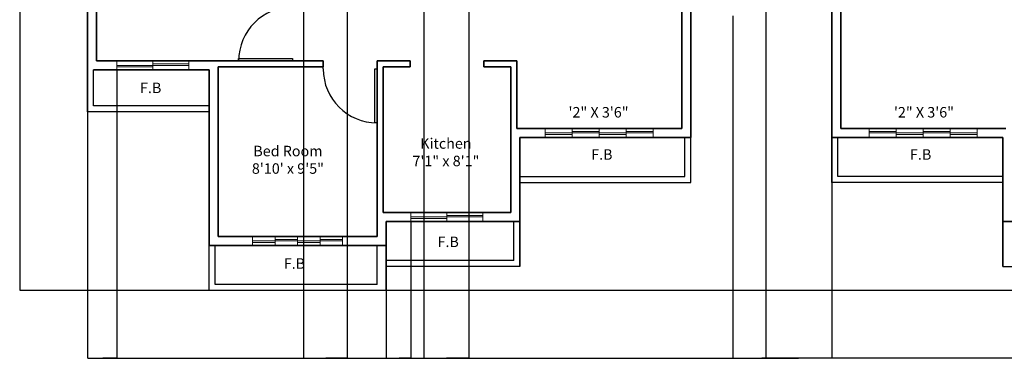
# Model space of a CAD drawing. Units: feet. Extents: x 105 to 1094, y -88 to 588.
# Tile 1 of 59: x 105 to 762, y -88 to 138. Entities that reach past the tile are written whole.
import ezdxf

# ---------------------------------------------------------------- set-up
doc = ezdxf.new("R2010")
doc.units = ezdxf.units.FT
doc.header["$MEASUREMENT"] = 0
for name, color, linetype, lineweight in [('A-ANNO-DIMS', 2, 'Continuous', 18), ('A-ANNO-TEXT', 7, 'Continuous', 18), ('A-AREA-IDEN', 7, 'Continuous', 18), ('A-DOOR', 3, 'Continuous', 25), ('A-FLOR-PROJ', 8, 'Continuous', 25), ('A-GLAZ', 4, 'Continuous', 18), ('A-WALL', 7, 'Continuous', 35)]:
    doc.layers.add(name, color=color, linetype=linetype, lineweight=lineweight)
doc.styles.get("Standard").update_dxf_attribs({"font": 'arial.ttf'})
doc.dimstyles.get("Standard").update_dxf_attribs({"dimtxt": 0.18, "dimasz": 0.18, "dimexe": 0.18, "dimexo": 0.0625, "dimgap": 0.09, "dimtad": 0, "dimtih": 1, "dimtoh": 1, "dimdec": 4, "dimzin": 0, "dimdsep": 46, "dimtxsty": 'Standard', "dimcen": 0.09, "dimadec": 0, "dimazin": 0, "dimtfac": 1, "dimtdec": 4, "dimtofl": 0, "dimtmove": 0, "dimatfit": 3, "dimfxl": 1, "dimtolj": 1, "dimtzin": 0, "dimarcsym": 0})

# ---------------------------------------------------------------- blocks, each defined once
blk = doc.blocks.new('*U2')
for p, q in [((0, 0), (0, -6)), ((40, 0), (40, -6))]:
    blk.add_line(p, q)
blk.add_lwpolyline([(0, 0), (0, 40), (1.75, 40), (1.75, 0)], close=True)
blk.add_arc((0, 0), 40, 0, 90)
blk = doc.blocks.new('WIN-FOUR-LIGHT-WIDE')
for p, q in [((0, 0), (0, 6)), ((0, 3), (72, 3)), ((0, 2), (18, 2)), ((18, 0), (18, 6)), ((18, 4), (36, 4)), ((36, 0), (36, 6)), ((36, 2), (54, 2)), ((54, 0), (54, 6)), ((54, 4), (72, 4)), ((72, 0), (72, 6))]:
    blk.add_line(p, q)
blk = doc.blocks.new('WIN-TWO-LIGHT')
for p, q in [((0, 0), (0, 6)), ((0, 3), (48, 3)), ((0, 2), (24, 2)), ((24, 0), (24, 6)), ((24, 4), (48, 4)), ((48, 0), (48, 6))]:
    blk.add_line(p, q)
blk = doc.blocks.new('WIN-FOUR-LIGHT')
for p, q in [((0, 0), (0, 6)), ((0, 3), (60, 3)), ((0, 2), (15, 2)), ((15, 0), (15, 6)), ((15, 4), (30, 4)), ((30, 0), (30, 6)), ((30, 2), (45, 2)), ((45, 0), (45, 6)), ((45, 4), (60, 4)), ((60, 0), (60, 6))]:
    blk.add_line(p, q)
blk = doc.blocks.new('*D20')
at = {"layer": 'A-ANNO-DIMS', "color": 0, "lineweight": -2, "transparency": 16777216}
for p, q in [((150.69, 276.02), (150.69, -88.15)), ((1048.69, 276.02), (1048.69, -88.15)), ((150.87, -87.97), (599.4, -87.97)), ((1048.51, -87.97), (599.98, -87.97))]:
    blk.add_line(p, q, dxfattribs=at)
at = {"layer": 'A-ANNO-DIMS', "color": 0, "transparency": 16777216}
for points in [[(150.87, -87.94), (150.87, -88), (150.69, -87.97)], [(1048.51, -87.94), (1048.51, -88), (1048.69, -87.97)]]:
    blk.add_solid(points, dxfattribs=at)
at = {"layer": 'Defpoints', "color": 0, "transparency": 16777216}
for p in [(150.69, 276.08), (1048.69, 276.08), (1048.69, -87.97)]:
    blk.add_point(p, dxfattribs=at)
at = {"layer": 'A-ANNO-DIMS', "color": 0, "transparency": 16777216, "insert": (599.69, -87.97), "char_height": 0.18, "attachment_point": 5}
blk.add_mtext('\\A1;898', dxfattribs=at)
blk = doc.blocks.new('*D21')
at = {"layer": 'A-ANNO-DIMS', "color": 0, "lineweight": -2, "transparency": 16777216}
for p, q in [((849.63, 543.08), (105.46, 543.08)), ((105.64, 542.9), (105.64, 250.26)), ((105.64, -42.74), (105.64, 249.9)), ((849.63, -42.92), (105.46, -42.92))]:
    blk.add_line(p, q, dxfattribs=at)
at = {"layer": 'A-ANNO-DIMS', "color": 0, "transparency": 16777216}
for points in [[(105.61, 542.9), (105.67, 542.9), (105.64, 543.08)], [(105.61, -42.74), (105.67, -42.74), (105.64, -42.92)]]:
    blk.add_solid(points, dxfattribs=at)
at = {"layer": 'Defpoints', "color": 0, "transparency": 16777216}
for p in [(105.64, 543.08), (849.69, 543.08), (849.69, -42.92)]:
    blk.add_point(p, dxfattribs=at)
at = {"layer": 'A-ANNO-DIMS', "color": 0, "transparency": 16777216, "insert": (105.64, 250.08), "char_height": 0.18, "attachment_point": 5}
blk.add_mtext('\\A1;586', dxfattribs=at)
blk = doc.blocks.new('*D35')
at = {"layer": 'A-ANNO-DIMS', "color": 0, "lineweight": -2, "transparency": 16777216}
for p, q in [((580.69, 140.02), (580.69, -88.15)), ((646.69, 140.02), (646.69, -88.15)), ((580.87, -87.97), (613.47, -87.97)), ((646.51, -87.97), (613.91, -87.97))]:
    blk.add_line(p, q, dxfattribs=at)
at = {"layer": 'A-ANNO-DIMS', "color": 0, "transparency": 16777216}
for points in [[(580.87, -87.94), (580.87, -88), (580.69, -87.97)], [(646.51, -87.94), (646.51, -88), (646.69, -87.97)]]:
    blk.add_solid(points, dxfattribs=at)
at = {"layer": 'Defpoints', "color": 0, "transparency": 16777216}
for p in [(580.69, 140.08), (646.69, 140.08), (646.69, -87.97)]:
    blk.add_point(p, dxfattribs=at)
at = {"layer": 'A-ANNO-DIMS', "color": 0, "transparency": 16777216, "insert": (613.69, -87.97), "char_height": 0.18, "attachment_point": 5}
blk.add_mtext('\\A1;66', dxfattribs=at)
blk = doc.blocks.new('*D37')
at = {"layer": 'A-ANNO-DIMS', "color": 0, "lineweight": -2, "transparency": 16777216}
for p, q in [((374.69, 150.53), (374.69, -88.15)), ((404.69, 150.02), (404.69, -88.15)), ((374.87, -87.97), (389.47, -87.97)), ((404.51, -87.97), (389.91, -87.97))]:
    blk.add_line(p, q, dxfattribs=at)
at = {"layer": 'A-ANNO-DIMS', "color": 0, "transparency": 16777216}
for points in [[(374.87, -87.94), (374.87, -88), (374.69, -87.97)], [(404.51, -87.94), (404.51, -88), (404.69, -87.97)]]:
    blk.add_solid(points, dxfattribs=at)
at = {"layer": 'Defpoints', "color": 0, "transparency": 16777216}
for p in [(374.69, 150.59), (404.69, 150.08), (404.69, -87.97)]:
    blk.add_point(p, dxfattribs=at)
at = {"layer": 'A-ANNO-DIMS', "color": 0, "transparency": 16777216, "insert": (389.69, -87.97), "char_height": 0.18, "attachment_point": 5}
blk.add_mtext('\\A1;30', dxfattribs=at)
blk = doc.blocks.new('*D40')
at = {"layer": 'A-ANNO-DIMS', "color": 0, "lineweight": -2, "transparency": 16777216}
for p, q in [((150.69, 106.02), (150.69, -88.15)), ((170.19, 104.02), (170.19, -88.15)), ((150.87, -87.97), (160.12, -87.97)), ((170.01, -87.97), (160.75, -87.97))]:
    blk.add_line(p, q, dxfattribs=at)
at = {"layer": 'A-ANNO-DIMS', "color": 0, "transparency": 16777216}
for points in [[(150.87, -87.94), (150.87, -88), (150.69, -87.97)], [(170.01, -87.94), (170.01, -88), (170.19, -87.97)]]:
    blk.add_solid(points, dxfattribs=at)
at = {"layer": 'Defpoints', "color": 0, "transparency": 16777216}
for p in [(150.69, 106.08), (170.19, 104.08), (170.19, -87.97)]:
    blk.add_point(p, dxfattribs=at)
at = {"layer": 'A-ANNO-DIMS', "color": 0, "transparency": 16777216, "insert": (160.44, -87.97), "char_height": 0.18, "attachment_point": 5}
blk.add_mtext('\\A1;19.5', dxfattribs=at)
blk = doc.blocks.new('*D43')
at = {"layer": 'A-ANNO-DIMS', "color": 0, "lineweight": -2, "transparency": 16777216}
for p, q in [((349.69, 3.02), (349.69, -88.15)), ((366.19, 3.02), (366.19, -88.15)), ((349.87, -87.97), (357.62, -87.97)), ((366.01, -87.97), (358.25, -87.97))]:
    blk.add_line(p, q, dxfattribs=at)
at = {"layer": 'A-ANNO-DIMS', "color": 0, "transparency": 16777216}
for points in [[(349.87, -87.94), (349.87, -88), (349.69, -87.97)], [(366.01, -87.94), (366.01, -88), (366.19, -87.97)]]:
    blk.add_solid(points, dxfattribs=at)
at = {"layer": 'Defpoints', "color": 0, "transparency": 16777216}
for p in [(349.69, 3.08), (366.19, 3.08), (366.19, -87.97)]:
    blk.add_point(p, dxfattribs=at)
at = {"layer": 'A-ANNO-DIMS', "color": 0, "transparency": 16777216, "insert": (357.94, -87.97), "char_height": 0.18, "attachment_point": 5}
blk.add_mtext('\\A1;16.5', dxfattribs=at)
blk = doc.blocks.new('*D44')
at = {"layer": 'A-ANNO-DIMS', "color": 0, "lineweight": -2, "transparency": 16777216}
for p, q in [((294.69, 204.02), (294.69, -88.15)), ((323.69, 204.02), (323.69, -88.15)), ((294.87, -87.97), (308.97, -87.97)), ((323.51, -87.97), (309.41, -87.97))]:
    blk.add_line(p, q, dxfattribs=at)
at = {"layer": 'A-ANNO-DIMS', "color": 0, "transparency": 16777216}
for points in [[(294.87, -87.94), (294.87, -88), (294.69, -87.97)], [(323.51, -87.94), (323.51, -88), (323.69, -87.97)]]:
    blk.add_solid(points, dxfattribs=at)
at = {"layer": 'Defpoints', "color": 0, "transparency": 16777216}
for p in [(294.69, 204.08), (323.69, 204.08), (323.69, -87.97)]:
    blk.add_point(p, dxfattribs=at)
at = {"layer": 'A-ANNO-DIMS', "color": 0, "transparency": 16777216, "insert": (309.19, -87.97), "char_height": 0.18, "attachment_point": 5}
blk.add_mtext('\\A1;29', dxfattribs=at)
blk = doc.blocks.new('*D49')
at = {"layer": 'A-ANNO-DIMS', "color": 0, "lineweight": -2, "transparency": 16777216}
for p, q in [((602.69, 295.02), (602.69, -88.15)), ((646.69, 295.02), (646.69, -88.15)), ((602.87, -87.97), (624.47, -87.97)), ((646.51, -87.97), (624.91, -87.97))]:
    blk.add_line(p, q, dxfattribs=at)
at = {"layer": 'A-ANNO-DIMS', "color": 0, "transparency": 16777216}
for points in [[(602.87, -87.94), (602.87, -88), (602.69, -87.97)], [(646.51, -87.94), (646.51, -88), (646.69, -87.97)]]:
    blk.add_solid(points, dxfattribs=at)
at = {"layer": 'Defpoints', "color": 0, "transparency": 16777216}
for p in [(602.69, 295.08), (646.69, 295.08), (646.69, -87.97)]:
    blk.add_point(p, dxfattribs=at)
at = {"layer": 'A-ANNO-DIMS', "color": 0, "transparency": 16777216, "insert": (624.69, -87.97), "char_height": 0.18, "attachment_point": 5}
blk.add_mtext('\\A1;44', dxfattribs=at)

msp = doc.modelspace()

# ---------------------------------------------------------------- linework, layer by layer
at = {"layer": 'A-FLOR-PROJ'}
for p, q in [((150.6883, 76.0812), (150.6883, 106.0812)), ((154.6883, 80.0812), (154.6883, 104.0812)), ((231.6883, 80.0812), (154.6883, 80.0812)), ((231.6883, 76.0812), (150.6883, 76.0812)), ((548.6883, 33.0812), (548.6883, 59.0812)), ((552.6883, 29.0812), (552.6883, 59.0812)), ((646.6883, 29.0812), (646.6883, 59.0812)), ((650.6883, 33.0812), (650.6883, 59.0812)), ((438.6883, 33.0812), (548.6883, 33.0812)), ((760.6883, 33.0812), (650.6883, 33.0812)), ((438.6883, 29.0812), (552.6883, 29.0812)), ((760.6883, 29.0812), (646.6883, 29.0812)), ((434.6883, -22.9188), (434.6883, 3.0812)), ((231.6883, -42.9188), (231.6883, -12.9188)), ((235.6883, -38.9188), (235.6883, -12.9188)), ((343.6883, -38.9188), (343.6883, -12.9188)), ((343.6883, -26.9188), (343.6883, -12.9188)), ((434.6883, -22.9188), (349.6883, -22.9188)), ((438.6883, -26.9188), (349.6883, -26.9188)), ((760.6883, -26.9188), (849.6883, -26.9188)), ((343.6883, -38.9188), (235.6883, -38.9188)), ((349.6883, -42.9188), (231.6883, -42.9188))]:
    msp.add_line(p, q, dxfattribs=at)
at = {"layer": 'A-WALL'}
for p, q in [((150.6883, 224.0812), (150.6883, 106.0812)), ((156.6883, 218.0812), (156.6883, 110.0812)), ((546.6883, 65.0812), (546.6883, 212.0812)), ((552.6883, 59.0812), (552.6883, 212.0812)), ((646.6883, 59.0812), (646.6883, 212.0812)), ((652.6883, 65.0812), (652.6883, 212.0812)), ((307.6883, 110.0812), (156.6883, 110.0812)), ((307.6883, 106.0812), (237.6883, 106.0812)), ((237.6883, -6.9188), (237.6883, 106.0812)), ((307.6883, 106.0812), (307.6883, 110.0812)), ((365.6883, 110.0812), (343.6883, 110.0812)), ((343.6883, -6.9188), (343.6883, 110.0812)), ((365.6883, 106.0812), (347.6883, 106.0812)), ((347.6883, 9.0812), (347.6883, 106.0812)), ((365.6883, 106.0812), (365.6883, 110.0812)), ((436.6883, 110.0812), (414.6883, 110.0812)), ((414.6883, 106.0812), (414.6883, 110.0812)), ((432.6883, 106.0812), (414.6883, 106.0812)), ((432.6883, 9.0812), (432.6883, 106.0812)), ((436.6883, 65.0812), (436.6883, 110.0812)), ((231.6883, 104.0812), (154.6883, 104.0812)), ((231.6883, -12.9188), (231.6883, 104.0812)), ((436.6883, 65.0812), (546.6883, 65.0812)), ((438.6883, 59.0812), (552.6883, 59.0812)), ((438.6883, -26.9188), (438.6883, 59.0812)), ((760.6883, 59.0812), (646.6883, 59.0812)), ((762.6883, 65.0812), (652.6883, 65.0812)), ((760.6883, -26.9188), (760.6883, 59.0812)), ((432.6883, 9.0812), (347.6883, 9.0812)), ((438.6883, 3.0812), (349.6883, 3.0812)), ((349.6883, -42.9188), (349.6883, 3.0812)), ((760.6883, 3.0812), (849.6883, 3.0812)), ((349.6883, -12.9188), (231.6883, -12.9188)), ((343.6883, -6.9188), (237.6883, -6.9188))]:
    msp.add_line(p, q, dxfattribs=at)

# ---------------------------------------------------------------- block references
at = {"layer": 'A-DOOR', "xscale": 0.8984622266767051, "yscale": 0.8984622266767051, "zscale": 0.8984622266767051}
for p, rotation in [((287.2975, 110.0812), 90.00000000000003), ((343.6883, 104.6904), 180)]:
    msp.add_blockref('*U2', p, dxfattribs=dict(at, rotation=rotation))
at = {"layer": 'A-GLAZ'}
for name, p in [('WIN-TWO-LIGHT', (170.188, 104.081)), ('WIN-FOUR-LIGHT-WIDE', (455.688, 59.081))]:
    msp.add_blockref(name, p, dxfattribs=at)
at = {"layer": 'A-GLAZ', "extrusion": (0, 0, -1), "zscale": -1}
msp.add_blockref('WIN-FOUR-LIGHT-WIDE', (-743.6886, 59.081), dxfattribs=at)
at = {"layer": 'A-GLAZ', "rotation": 180}
for name, p in [('WIN-TWO-LIGHT', (414.1886, 9.0813)), ('WIN-FOUR-LIGHT', (320.6886, -6.9187))]:
    msp.add_blockref(name, p, dxfattribs=at)

# ---------------------------------------------------------------- texts
at = {"layer": 'A-ANNO-DIMS', "char_height": 7}
for insert, attachment_point in [((540.4102, 72.3375), 9), ((658.9665, 72.3375), 7)]:
    msp.add_mtext_dynamic_manual_height_columns('\\pxqc;\'2" X 3\'6"', width=98.34246, gutter_width=1, heights=[0], dxfattribs=dict(at, insert=insert, attachment_point=attachment_point))
at = {"layer": 'A-ANNO-TEXT', "char_height": 7}
for insert, attachment_point in [((241.9039, 88.6015), 9), ((542.6156, 44.1875), 9), ((656.7611, 44.1875), 7), ((440.205, -14.01), 9), ((337.7459, -28.4972), 9)]:
    msp.add_mtext_dynamic_manual_height_columns('\\pxqc;F.B ', width=98.34246, gutter_width=1, heights=[0], dxfattribs=dict(at, insert=insert, attachment_point=attachment_point))
at = {"layer": 'A-AREA-IDEN', "char_height": 7, "attachment_point": 9}
for s, insert in [('\\pxqc;Kitchen  \\P7\'1" x 8\'1"', (438.6883, 39.8597)), ('\\pxqc;Bed Room \\P8\'10\' x 9\'5"', (333.3837, 34.8333))]:
    msp.add_mtext_dynamic_manual_height_columns(s, width=98.34246, gutter_width=1, heights=[0], dxfattribs=dict(at, insert=insert))

# ---------------------------------------------------------------- dimensions: what is measured, and where the dimension line sits
at = {"layer": 'A-ANNO-DIMS'}
dim = msp.add_linear_dim(base=(105.6383, 543.0812), p1=(849.6883, -42.9188), p2=(849.6883, 543.0812), angle=90, dimstyle='Standard', override={"dimdec": 0, "dimlfac": 1, "dimrnd": 0, "dimzin": 0, "dimdsep": 46, "dimlunit": 2}, dxfattribs=at)
dim.commit()
dim.dimension.update_dxf_attribs({"geometry": '*D21', "text_midpoint": (105.6383, 250.0812)})
for base, p1, p2, override, picture, middle in [((646.6883, -87.9688), (602.6883, 295.0812), (646.6883, 295.0812), {"dimdec": 0, "dimlfac": 1, "dimrnd": 0, "dimzin": 0, "dimdsep": 46, "dimlunit": 2}, '*D49', (624.6883, -87.9688)), ((1048.6883, -87.9688), (150.6883, 276.0812), (1048.6883, 276.0812), {"dimdec": 0, "dimlfac": 1, "dimrnd": 0, "dimzin": 0, "dimdsep": 46, "dimlunit": 2}, '*D20', (599.6883, -87.9688)), ((323.6883, -87.9688), (294.6883, 204.0812), (323.6883, 204.0812), {"dimdec": 0, "dimlfac": 1, "dimrnd": 0, "dimzin": 0, "dimdsep": 46, "dimlunit": 2}, '*D44', (309.1883, -87.9688)), ((404.6883, -87.9688), (374.6883, 150.5895), (404.6883, 150.0812), {"dimdec": 0, "dimlfac": 1, "dimrnd": 0, "dimzin": 0, "dimdsep": 46, "dimlunit": 2}, '*D37', (389.6883, -87.9688)), ((646.6883, -87.9688), (580.6883, 140.0812), (646.6883, 140.0812), {"dimdec": 0, "dimlfac": 1, "dimrnd": 0, "dimzin": 0, "dimdsep": 46, "dimlunit": 2}, '*D35', (613.6883, -87.9688)), ((170.1883, -87.9688), (150.6883, 106.0812), (170.1883, 104.0812), {"dimdec": 1, "dimlfac": 1, "dimrnd": 0, "dimzin": 0, "dimdsep": 46, "dimlunit": 2}, '*D40', (160.4383, -87.9688)), ((366.1883, -87.9688), (349.6883, 3.0812), (366.1883, 3.0812), {"dimdec": 1, "dimlfac": 1, "dimrnd": 0, "dimzin": 0, "dimdsep": 46, "dimlunit": 2}, '*D43', (357.9383, -87.9688))]:
    dim = msp.add_linear_dim(base=base, p1=p1, p2=p2, dimstyle='Standard', override=override, dxfattribs=at)
    dim.commit()
    dim.dimension.update_dxf_attribs({"geometry": picture, "text_midpoint": middle})

doc.saveas('drawing.dxf')
